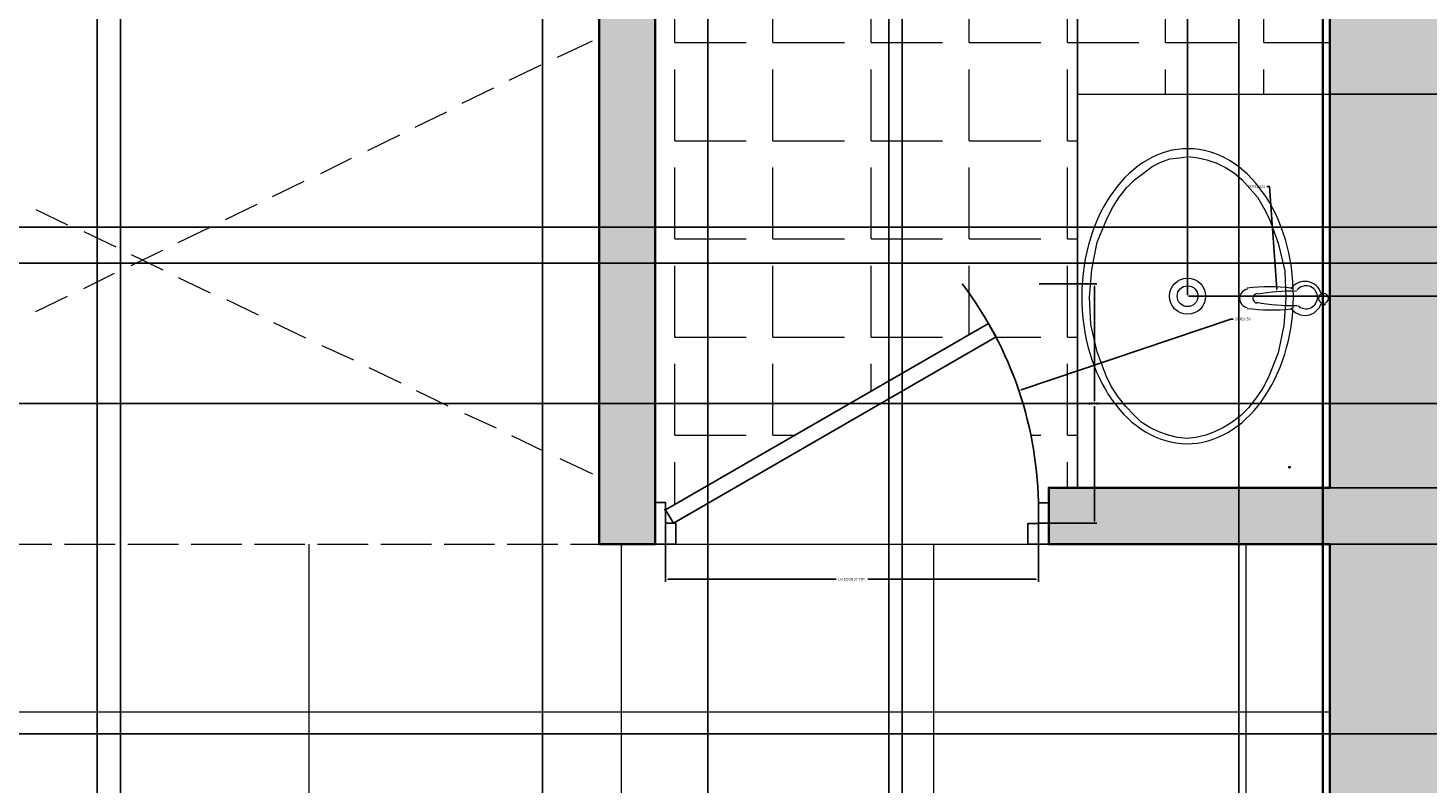
# Model space of a CAD drawing. Units: inches. Extents: x 6 to 575, y 34 to 566.
# Tile 17 of 21: x 282 to 382, y 432 to 486. Entities that reach past the tile are written whole.
import ezdxf

# ---------------------------------------------------------------- set-up
doc = ezdxf.new("R2010")
doc.units = ezdxf.units.IN
doc.linetypes.add('ACAD_ISO02W100', pattern=[15, 12, -3])
for name, color, linetype, lineweight in [('A-ANNO-DIMS', 2, 'Continuous', 18), ('A-FLOR-CASE', 2, 'Continuous', 18), ('A-FLOR-FIXT', 9, 'Continuous', 18), ('A-FLOR-PATT', 252, 'Continuous', 9), ('A-FLOR-STRS-OVHD', 1, 'ACAD_ISO02W100', 13), ('A-WALL-PATT', 251, 'Continuous', 9), ('DOORS', 3, 'Continuous', 25), ('STAIRS', 1, 'Continuous', 20), ('WALLS', 7, 'Continuous', 35)]:
    doc.layers.add(name, color=color, linetype=linetype, lineweight=lineweight)
doc.styles.get("Standard").update_dxf_attribs({"font": 'arial.ttf'})
doc.dimstyles.get("Standard").update_dxf_attribs({"dimtxt": 0.18, "dimasz": 0.18, "dimexe": 0.18, "dimexo": 0.0625, "dimgap": 0.09, "dimtad": 0, "dimtih": 1, "dimtoh": 1, "dimdec": 4, "dimzin": 0, "dimdsep": 46, "dimtxsty": 'Standard', "dimcen": 0.09, "dimadec": 0, "dimazin": 0, "dimtfac": 1, "dimtdec": 4, "dimtofl": 0, "dimtmove": 0, "dimatfit": 3, "dimfxl": 1, "dimtolj": 1, "dimtzin": 0, "dimarcsym": 0})

# ---------------------------------------------------------------- blocks, each defined once
blk = doc.blocks.new('Door - Left Hung 36 in.')
blk.add_lwpolyline([(0.75, -1.3), (0, 0), (31.18, 18), (31.93, 16.7)], close=True)
blk.add_arc((0, 0), 36, 0, 37.3101)
blk = doc.blocks.new('*D13')
at = {"layer": 'A-ANNO-DIMS', "color": 0, "lineweight": -2, "transparency": 16777216}
for p, q in [((327.396, 450.212), (327.396, 446.115)), ((353.927, 450.212), (353.927, 446.115)), ((327.576, 446.295), (339.529, 446.295)), ((353.747, 446.295), (341.793, 446.295))]:
    blk.add_line(p, q, dxfattribs=at)
at = {"layer": 'A-ANNO-DIMS', "color": 0, "transparency": 16777216}
for points in [[(327.576, 446.325), (327.576, 446.265), (327.396, 446.295)], [(353.747, 446.325), (353.747, 446.265), (353.927, 446.295)]]:
    blk.add_solid(points, dxfattribs=at)
at = {"layer": 'Defpoints', "color": 0, "transparency": 16777216}
for p in [(327.396, 450.275), (353.927, 450.275), (353.927, 446.295)]:
    blk.add_point(p, dxfattribs=at)
at = {"layer": 'A-ANNO-DIMS', "color": 0, "transparency": 16777216, "insert": (340.661, 446.295), "char_height": 0.18, "attachment_point": 5}
blk.add_mtext('\\A1;LH DOOR 27 TYP.', dxfattribs=at)
blk = doc.blocks.new('*D14')
at = {"layer": 'A-ANNO-DIMS', "color": 0, "lineweight": -2, "transparency": 16777216}
for p, q in [((353.989, 467.313), (358.086, 467.313)), ((357.906, 467.133), (357.906, 458.975)), ((357.906, 450.455), (357.906, 458.614)), ((353.989, 450.275), (358.086, 450.275))]:
    blk.add_line(p, q, dxfattribs=at)
at = {"layer": 'A-ANNO-DIMS', "color": 0, "transparency": 16777216}
for points in [[(357.876, 467.133), (357.936, 467.133), (357.906, 467.313)], [(357.876, 450.455), (357.936, 450.455), (357.906, 450.275)]]:
    blk.add_solid(points, dxfattribs=at)
at = {"layer": 'Defpoints', "color": 0, "transparency": 16777216}
for p in [(353.927, 467.313), (357.906, 467.313), (353.927, 450.275)]:
    blk.add_point(p, dxfattribs=at)
at = {"layer": 'A-ANNO-DIMS', "color": 0, "transparency": 16777216, "insert": (357.906, 458.794), "char_height": 0.18, "attachment_point": 5}
blk.add_mtext('\\A1;17 TYP.', dxfattribs=at)
blk = doc.blocks.new('*D50')
at = {"layer": 'A-ANNO-DIMS', "color": 0, "lineweight": -2, "transparency": 16777216}
for p, q in [((248.696, 468.775), (574.676, 468.775)), ((574.496, 468.595), (574.496, 463.964)), ((574.496, 458.969), (574.496, 463.6)), ((248.696, 458.789), (574.676, 458.789))]:
    blk.add_line(p, q, dxfattribs=at)
at = {"layer": 'A-ANNO-DIMS', "color": 0, "transparency": 16777216}
for points in [[(574.466, 468.595), (574.526, 468.595), (574.496, 468.775)], [(574.466, 458.969), (574.526, 458.969), (574.496, 458.789)]]:
    blk.add_solid(points, dxfattribs=at)
at = {"layer": 'Defpoints', "color": 0, "transparency": 16777216}
for p in [(248.633, 468.775), (574.496, 468.775), (248.633, 458.789)]:
    blk.add_point(p, dxfattribs=at)
at = {"layer": 'A-ANNO-DIMS', "color": 0, "transparency": 16777216, "insert": (574.496, 463.782), "char_height": 0.18, "attachment_point": 5}
blk.add_mtext('\\A1;9.987', dxfattribs=at)
blk = doc.blocks.new('*D52')
at = {"layer": 'A-ANNO-DIMS', "color": 0, "lineweight": -2, "transparency": 16777216}
for p, q in [((437.624, 471.353), (6.649, 471.353)), ((6.829, 471.173), (6.829, 453.513)), ((6.829, 435.488), (6.829, 453.149)), ((437.624, 435.308), (6.649, 435.308))]:
    blk.add_line(p, q, dxfattribs=at)
at = {"layer": 'A-ANNO-DIMS', "color": 0, "transparency": 16777216}
for points in [[(6.799, 471.173), (6.859, 471.173), (6.829, 471.353)], [(6.799, 435.488), (6.859, 435.488), (6.829, 435.308)]]:
    blk.add_solid(points, dxfattribs=at)
at = {"layer": 'Defpoints', "color": 0, "transparency": 16777216}
for p in [(6.829, 471.353), (437.687, 471.353), (437.687, 435.308)]:
    blk.add_point(p, dxfattribs=at)
at = {"layer": 'A-ANNO-DIMS', "color": 0, "transparency": 16777216, "insert": (6.829, 453.331), "char_height": 0.18, "attachment_point": 5}
blk.add_mtext('\\A1;36.045', dxfattribs=at)
blk = doc.blocks.new('*D63')
at = {"layer": 'A-ANNO-DIMS', "color": 0, "lineweight": -2, "transparency": 16777216}
for p, q in [((322.659, 448.863), (322.659, 565.811)), ((322.839, 565.631), (324.506, 565.631)), ((326.479, 565.631), (324.811, 565.631)), ((326.659, 448.863), (326.659, 565.811))]:
    blk.add_line(p, q, dxfattribs=at)
at = {"layer": 'A-ANNO-DIMS', "color": 0, "transparency": 16777216}
for points in [[(322.839, 565.661), (322.839, 565.601), (322.659, 565.631)], [(326.479, 565.661), (326.479, 565.601), (326.659, 565.631)]]:
    blk.add_solid(points, dxfattribs=at)
at = {"layer": 'Defpoints', "color": 0, "transparency": 16777216}
for p in [(326.659, 565.631), (322.659, 448.801), (326.659, 448.801)]:
    blk.add_point(p, dxfattribs=at)
at = {"layer": 'A-ANNO-DIMS', "color": 0, "transparency": 16777216, "insert": (324.659, 565.631), "char_height": 0.18, "attachment_point": 5}
blk.add_mtext('\\A1;4', dxfattribs=at)
blk = doc.blocks.new('*D64')
at = {"layer": 'A-ANNO-DIMS', "color": 0, "lineweight": -2, "transparency": 16777216}
for p, q in [((354.721145, 452.800984), (574.675816, 452.800984)), ((574.495816, 452.620984), (574.495816, 450.980984)), ((574.495816, 448.980984), (574.495816, 450.620984)), ((354.721145, 448.800984), (574.675816, 448.800984))]:
    blk.add_line(p, q, dxfattribs=at)
at = {"layer": 'A-ANNO-DIMS', "color": 0, "transparency": 16777216}
for points in [[(574.465816, 452.620984), (574.525816, 452.620984), (574.495816, 452.800984)], [(574.465816, 448.980984), (574.525816, 448.980984), (574.495816, 448.800984)]]:
    blk.add_solid(points, dxfattribs=at)
at = {"layer": 'Defpoints', "color": 0, "transparency": 16777216}
for p in [(354.658645, 452.800984), (574.495816, 452.800984), (354.658645, 448.800984)]:
    blk.add_point(p, dxfattribs=at)
at = {"layer": 'A-ANNO-DIMS', "color": 0, "transparency": 16777216, "insert": (574.495816, 450.800984), "char_height": 0.18, "attachment_point": 5}
blk.add_mtext('\\A1;4', dxfattribs=at)
blk = doc.blocks.new('*D73')
at = {"layer": 'A-ANNO-DIMS', "color": 0, "lineweight": -2, "transparency": 16777216}
for p, q in [((248.633, 448.865), (248.633, 565.811)), ((248.813, 565.631), (285.253, 565.631)), ((322.479, 565.631), (286.039, 565.631)), ((322.659, 448.863), (322.659, 565.811))]:
    blk.add_line(p, q, dxfattribs=at)
at = {"layer": 'A-ANNO-DIMS', "color": 0, "transparency": 16777216}
for points in [[(248.813, 565.661), (248.813, 565.601), (248.633, 565.631)], [(322.479, 565.661), (322.479, 565.601), (322.659, 565.631)]]:
    blk.add_solid(points, dxfattribs=at)
at = {"layer": 'Defpoints', "color": 0, "transparency": 16777216}
for p in [(322.659, 565.631), (248.633, 448.802), (322.659, 448.801)]:
    blk.add_point(p, dxfattribs=at)
at = {"layer": 'A-ANNO-DIMS', "color": 0, "transparency": 16777216, "insert": (285.646, 565.631), "char_height": 0.18, "attachment_point": 5}
blk.add_mtext('\\A1;74.03', dxfattribs=at)
blk = doc.blocks.new('*D119')
at = {"layer": 'A-ANNO-DIMS', "color": 0, "lineweight": -2, "transparency": 16777216}
for p, q in [((343.278, 400.02), (343.278, 565.811)), ((343.458, 565.631), (358.358, 565.631)), ((374.011, 565.631), (359.111, 565.631)), ((374.191, 395.441), (374.191, 565.811))]:
    blk.add_line(p, q, dxfattribs=at)
at = {"layer": 'A-ANNO-DIMS', "color": 0, "transparency": 16777216}
for points in [[(343.458, 565.661), (343.458, 565.601), (343.278, 565.631)], [(374.011, 565.661), (374.011, 565.601), (374.191, 565.631)]]:
    blk.add_solid(points, dxfattribs=at)
at = {"layer": 'Defpoints', "color": 0, "transparency": 16777216}
for p in [(374.191, 565.631), (343.278, 399.958), (374.191, 395.379)]:
    blk.add_point(p, dxfattribs=at)
at = {"layer": 'A-ANNO-DIMS', "color": 0, "transparency": 16777216, "insert": (358.734, 565.631), "char_height": 0.18, "attachment_point": 5}
blk.add_mtext('\\A1;30.91', dxfattribs=at)
blk = doc.blocks.new('*D126')
at = {"layer": 'A-ANNO-DIMS', "color": 0, "lineweight": -2, "transparency": 16777216}
for p, q in [((368.183, 318.514), (368.183, 565.811)), ((368.363, 565.631), (370.782, 565.631)), ((373.954, 565.631), (371.535, 565.631)), ((374.134, 318.458), (374.134, 565.811))]:
    blk.add_line(p, q, dxfattribs=at)
at = {"layer": 'A-ANNO-DIMS', "color": 0, "transparency": 16777216}
for points in [[(368.363, 565.661), (368.363, 565.601), (368.183, 565.631)], [(373.954, 565.661), (373.954, 565.601), (374.134, 565.631)]]:
    blk.add_solid(points, dxfattribs=at)
at = {"layer": 'Defpoints', "color": 0, "transparency": 16777216}
for p in [(374.134, 565.631), (368.183, 318.451), (374.134, 318.395)]:
    blk.add_point(p, dxfattribs=at)
at = {"layer": 'A-ANNO-DIMS', "color": 0, "transparency": 16777216, "insert": (371.158, 565.631), "char_height": 0.18, "attachment_point": 5}
blk.add_mtext('\\A1;5.951', dxfattribs=at)
blk = doc.blocks.new('*D127')
at = {"layer": 'A-ANNO-DIMS', "color": 0, "lineweight": -2, "transparency": 16777216}
for p, q in [((286.946, 310.606), (286.946, 565.811)), ((287.126, 565.631), (308.278, 565.631)), ((330.225, 565.631), (309.073, 565.631)), ((330.405, 310.606), (330.405, 565.811))]:
    blk.add_line(p, q, dxfattribs=at)
at = {"layer": 'A-ANNO-DIMS', "color": 0, "transparency": 16777216}
for points in [[(287.126, 565.661), (287.126, 565.601), (286.946, 565.631)], [(330.225, 565.661), (330.225, 565.601), (330.405, 565.631)]]:
    blk.add_solid(points, dxfattribs=at)
at = {"layer": 'Defpoints', "color": 0, "transparency": 16777216}
for p in [(330.405, 565.631), (286.946, 310.543), (330.405, 310.543)]:
    blk.add_point(p, dxfattribs=at)
at = {"layer": 'A-ANNO-DIMS', "color": 0, "transparency": 16777216, "insert": (308.675, 565.631), "char_height": 0.18, "attachment_point": 5}
blk.add_mtext('\\A1;43.46', dxfattribs=at)
blk = doc.blocks.new('*D129')
at = {"layer": 'A-ANNO-DIMS', "color": 0, "lineweight": -2, "transparency": 16777216}
for p, q in [((330.405, 310.606), (330.405, 565.811)), ((330.585, 565.631), (336.387, 565.631)), ((343.098, 565.631), (337.296, 565.631)), ((343.278, 313.883), (343.278, 565.811))]:
    blk.add_line(p, q, dxfattribs=at)
at = {"layer": 'A-ANNO-DIMS', "color": 0, "transparency": 16777216}
for points in [[(330.585, 565.661), (330.585, 565.601), (330.405, 565.631)], [(343.098, 565.661), (343.098, 565.601), (343.278, 565.631)]]:
    blk.add_solid(points, dxfattribs=at)
at = {"layer": 'Defpoints', "color": 0, "transparency": 16777216}
for p in [(343.278, 565.631), (343.278, 313.82), (330.405, 310.543)]:
    blk.add_point(p, dxfattribs=at)
at = {"layer": 'A-ANNO-DIMS', "color": 0, "transparency": 16777216, "insert": (336.841, 565.631), "char_height": 0.18, "attachment_point": 5}
blk.add_mtext('\\A1;12.874', dxfattribs=at)
blk = doc.blocks.new('*D131')
at = {"layer": 'A-ANNO-DIMS', "color": 0, "lineweight": -2, "transparency": 16777216}
for p, q in [((288.603, 342.076), (288.603, 565.811)), ((288.783, 565.631), (303.229, 565.631)), ((318.461, 565.631), (304.015, 565.631)), ((318.641, 342.076), (318.641, 565.811))]:
    blk.add_line(p, q, dxfattribs=at)
at = {"layer": 'A-ANNO-DIMS', "color": 0, "transparency": 16777216}
for points in [[(288.783, 565.661), (288.783, 565.601), (288.603, 565.631)], [(318.461, 565.661), (318.461, 565.601), (318.641, 565.631)]]:
    blk.add_solid(points, dxfattribs=at)
at = {"layer": 'Defpoints', "color": 0, "transparency": 16777216}
for p in [(318.641, 565.631), (288.603, 342.013), (318.641, 342.013)]:
    blk.add_point(p, dxfattribs=at)
at = {"layer": 'A-ANNO-DIMS', "color": 0, "transparency": 16777216, "insert": (303.622, 565.631), "char_height": 0.18, "attachment_point": 5}
blk.add_mtext('\\A1;30.04', dxfattribs=at)
blk = doc.blocks.new('*D134')
at = {"layer": 'A-ANNO-DIMS', "color": 0, "lineweight": -2, "transparency": 16777216}
for p, q in [((318.641, 342.076), (318.641, 565.811)), ((318.821, 565.631), (331.04, 565.631)), ((344.051, 565.631), (331.831, 565.631)), ((344.231, 343.012), (344.231, 565.811))]:
    blk.add_line(p, q, dxfattribs=at)
at = {"layer": 'A-ANNO-DIMS', "color": 0, "transparency": 16777216}
for points in [[(318.821, 565.661), (318.821, 565.601), (318.641, 565.631)], [(344.051, 565.661), (344.051, 565.601), (344.231, 565.631)]]:
    blk.add_solid(points, dxfattribs=at)
at = {"layer": 'Defpoints', "color": 0, "transparency": 16777216}
for p in [(344.231, 565.631), (344.231, 342.949), (318.641, 342.013)]:
    blk.add_point(p, dxfattribs=at)
at = {"layer": 'A-ANNO-DIMS', "color": 0, "transparency": 16777216, "insert": (331.436, 565.631), "char_height": 0.18, "attachment_point": 5}
blk.add_mtext('\\A1;25.59', dxfattribs=at)
blk = doc.blocks.new('*D193')
at = {"layer": 'A-ANNO-DIMS', "color": 0, "lineweight": -2, "transparency": 16777216}
for p, q in [((356.714, 452.863), (356.714, 565.811)), ((356.894, 565.631), (365.231, 565.631)), ((374.479, 565.631), (366.142, 565.631)), ((374.659, 480.873), (374.659, 565.811))]:
    blk.add_line(p, q, dxfattribs=at)
at = {"layer": 'A-ANNO-DIMS', "color": 0, "transparency": 16777216}
for points in [[(356.894, 565.661), (356.894, 565.601), (356.714, 565.631)], [(374.479, 565.661), (374.479, 565.601), (374.659, 565.631)]]:
    blk.add_solid(points, dxfattribs=at)
at = {"layer": 'Defpoints', "color": 0, "transparency": 16777216}
for p in [(374.659, 565.631), (374.659, 480.81), (356.714, 452.801)]:
    blk.add_point(p, dxfattribs=at)
at = {"layer": 'A-ANNO-DIMS', "color": 0, "transparency": 16777216, "insert": (365.686, 565.631), "char_height": 0.18, "attachment_point": 5}
blk.add_mtext('\\A1;17.945', dxfattribs=at)
blk = doc.blocks.new('*D194')
at = {"layer": 'A-ANNO-DIMS', "color": 0, "lineweight": -2, "transparency": 16777216}
for p, q in [((374.721, 480.81), (574.676, 480.81)), ((574.496, 480.63), (574.496, 466.987)), ((574.496, 452.981), (574.496, 466.624)), ((356.777, 452.801), (574.676, 452.801))]:
    blk.add_line(p, q, dxfattribs=at)
at = {"layer": 'A-ANNO-DIMS', "color": 0, "transparency": 16777216}
for points in [[(574.466, 480.63), (574.526, 480.63), (574.496, 480.81)], [(574.466, 452.981), (574.526, 452.981), (574.496, 452.801)]]:
    blk.add_solid(points, dxfattribs=at)
at = {"layer": 'Defpoints', "color": 0, "transparency": 16777216}
for p in [(374.659, 480.81), (574.496, 480.81), (356.714, 452.801)]:
    blk.add_point(p, dxfattribs=at)
at = {"layer": 'A-ANNO-DIMS', "color": 0, "transparency": 16777216, "insert": (574.496, 466.806), "char_height": 0.18, "attachment_point": 5}
blk.add_mtext('\\A1;28.01', dxfattribs=at)
blk = doc.blocks.new('*D195')
at = {"layer": 'A-ANNO-DIMS', "color": 0, "lineweight": -2, "transparency": 16777216}
for p, q in [((364.602, 466.433), (574.676, 466.433)), ((574.496, 466.253), (574.496, 459.799)), ((574.496, 452.981), (574.496, 459.435)), ((374.721, 452.801), (574.676, 452.801))]:
    blk.add_line(p, q, dxfattribs=at)
at = {"layer": 'A-ANNO-DIMS', "color": 0, "transparency": 16777216}
for points in [[(574.466, 466.253), (574.526, 466.253), (574.496, 466.433)], [(574.466, 452.981), (574.526, 452.981), (574.496, 452.801)]]:
    blk.add_solid(points, dxfattribs=at)
at = {"layer": 'Defpoints', "color": 0, "transparency": 16777216}
for p in [(364.54, 466.433), (574.496, 466.433), (374.659, 452.801)]:
    blk.add_point(p, dxfattribs=at)
at = {"layer": 'A-ANNO-DIMS', "color": 0, "transparency": 16777216, "insert": (574.496, 459.617), "char_height": 0.18, "attachment_point": 5}
blk.add_mtext('\\A1;13.632', dxfattribs=at)
blk = doc.blocks.new('*D196')
at = {"layer": 'A-ANNO-DIMS', "color": 0, "lineweight": -2, "transparency": 16777216}
for p, q in [((364.54, 466.496), (364.54, 565.811)), ((364.72, 565.631), (369.215, 565.631)), ((374.479, 565.631), (369.983, 565.631)), ((374.659, 452.863), (374.659, 565.811))]:
    blk.add_line(p, q, dxfattribs=at)
at = {"layer": 'A-ANNO-DIMS', "color": 0, "transparency": 16777216}
for points in [[(364.72, 565.661), (364.72, 565.601), (364.54, 565.631)], [(374.479, 565.661), (374.479, 565.601), (374.659, 565.631)]]:
    blk.add_solid(points, dxfattribs=at)
at = {"layer": 'Defpoints', "color": 0, "transparency": 16777216}
for p in [(364.54, 565.631), (364.54, 466.433), (374.659, 452.801)]:
    blk.add_point(p, dxfattribs=at)
at = {"layer": 'A-ANNO-DIMS', "color": 0, "transparency": 16777216, "insert": (369.599, 565.631), "char_height": 0.18, "attachment_point": 5}
blk.add_mtext('\\A1;10.12', dxfattribs=at)
blk = doc.blocks.new('*D230')
at = {"layer": 'A-ANNO-DIMS', "color": 0, "lineweight": -2, "transparency": 16777216}
for p, q in [((367.615, 464.811), (352.703, 459.776)), ((367.795, 464.811), (367.615, 464.811)), ((327.396, 451.142), (327.396, 451.322)), ((327.306, 451.232), (327.486, 451.232))]:
    blk.add_line(p, q, dxfattribs=at)
at = {"layer": 'A-ANNO-DIMS', "color": 0, "transparency": 16777216}
blk.add_solid([(352.694, 459.805), (352.713, 459.748), (352.533, 459.719)], dxfattribs=at)
at = {"layer": 'Defpoints', "color": 0, "transparency": 16777216}
for p in [(352.533, 459.719), (327.396, 451.232)]:
    blk.add_point(p, dxfattribs=at)
at = {"layer": 'A-ANNO-DIMS', "color": 0, "transparency": 16777216, "insert": (368.47, 464.811), "char_height": 0.18, "attachment_point": 5}
blk.add_mtext('\\A1;2X R26.53', dxfattribs=at)
blk = doc.blocks.new('*D233')
at = {"layer": 'A-ANNO-DIMS', "color": 0, "lineweight": -2, "transparency": 16777216}
for p, q in [((370.184, 474.246), (370.364, 474.246)), ((370.364, 474.246), (370.888, 466.931)), ((371.796, 454.172), (371.796, 454.352)), ((371.706, 454.262), (371.886, 454.262))]:
    blk.add_line(p, q, dxfattribs=at)
at = {"layer": 'A-ANNO-DIMS', "color": 0, "transparency": 16777216}
blk.add_solid([(370.918, 466.934), (370.858, 466.929), (370.901, 466.752)], dxfattribs=at)
at = {"layer": 'Defpoints', "color": 0, "transparency": 16777216}
for p in [(370.901, 466.752), (371.796, 454.262)]:
    blk.add_point(p, dxfattribs=at)
at = {"layer": 'A-ANNO-DIMS', "color": 0, "transparency": 16777216, "insert": (369.44, 474.246), "char_height": 0.18, "attachment_point": 5}
blk.add_mtext('\\A1;2X R12.522', dxfattribs=at)

msp = doc.modelspace()

# ---------------------------------------------------------------- hatches: boundary and pattern name
at = {"layer": 'A-FLOR-PATT'}
h = msp.add_hatch(dxfattribs=at)
h.set_pattern_fill('ANGLE', color=256)
h.set_pattern_definition([(0, (-98.035, 170.1465), (0, 6.985), [5.08, -1.905]), (90, (-98.035, 170.1465), (-6.985, 4e-16), [5.08, -1.905])])
h.paths.add_polyline_path([(374.6586, 530.801), (362.6586, 530.801), (338.6586, 530.801), (326.6586, 530.801), (326.6586, 451.7489), (327.3956, 451.7489), (327.3956, 451.2323), (350.3721, 464.4978), (350.9248, 463.5404), (350.9049, 463.5289, -0.1161983), (353.9217, 451.7417), (354.6586, 451.7417), (354.6586, 452.801), (356.7141, 452.801), (356.7141, 480.81), (374.6586, 480.81)])
h = msp.add_hatch(dxfattribs=at)
h.set_pattern_fill('NET', color=256, scale=7)
h.set_pattern_definition([(0, (-98.035, 170.147), (0, 22.225), []), (90, (-98.035, 170.147), (-22.225, 1e-15), [])])
h.paths.add_polyline_path([(368.183, 395.6385, -0.8837053), (374.2533, 394.8861), (374.6586, 448.801), (354.6586, 448.801), (354.6586, 448.7938), (353.1847, 448.7938), (326.6586, 448.801), (322.6586, 448.801), (248.6332, 448.8024), (206.6586, 448.8024), (206.6586, 389.449), (221.6622, 389.449), (221.6622, 310.5712), (206.6586, 310.5712), (206.6586, 276.801), (206.6704, 276.801), (206.6704, 274.3795), (206.6586, 224.801), (246.6586, 224.801), (264.6586, 224.801), (265.6986, 224.801), (265.6986, 249.081), (267.5186, 249.081), (267.5186, 249.0145, -0.3851529), (290.6494, 224.801), (290.6679, 224.801, -0.3851529), (313.7986, 249.0145), (313.7986, 249.081), (315.6186, 249.081), (315.6186, 224.801), (316.6586, 224.801), (334.6586, 224.801), (374.6586, 224.801), (374.6586, 278.801), (374.1753, 318.8919, -0.4553029), (370.7577, 315.9168), (370.6643, 313.8205, -0.4142136), (368.7528, 311.909), (368.8072, 311.8975), (368.7528, 311.909, 0.4142136), (370.6643, 313.8205), (370.7632, 315.9161, -0.346346), (368.183, 318.5897)])
h.paths.add_polyline_path([(288.603, 342.0131), (288.603, 389.9952), (318.6406, 389.9952), (318.6406, 342.0131)], flags=16)
h.paths.add_polyline_path([(289.6173, 343.0274), (289.6173, 389.059), (317.6263, 389.059), (317.6263, 343.0274)], flags=0)
h.paths.add_polyline_path([(295.4867, 311.7535, 0.0653816), (295.1241, 312.0945), (295.0006, 312.1316)], flags=16)
h.paths.add_polyline_path([(328.4931, 284.9911, 0.4142136), (330.4045, 286.9026), (330.4215, 286.8532), (330.4045, 286.9026, -0.4142136), (328.4931, 284.9911), (328.549, 284.9808)], flags=16)
h.paths.add_polyline_path([(344.7771, 305.2659), (368.8072, 305.2659), (368.8072, 281.2358), (344.7771, 281.2358)], flags=16)
h.paths.add_polyline_path([(368.183, 288.1406, -1), (356.246, 288.1406, -1)], flags=0)
h.paths.add_polyline_path([(347.9759, 404.6629), (347.9759, 428.6929), (372.006, 428.6929), (372.006, 404.6629)], flags=16)
h.paths.add_polyline_path([(359.4448, 421.7882, -1), (371.3818, 421.7882, -1)], flags=0)
at = {"layer": 'A-WALL-PATT'}
h = msp.add_hatch(color=256, dxfattribs=at)
h.dxf.hatch_style = 1
h.paths.add_polyline_path([(160.6586, 539.801), (32.6586, 539.801), (32.6586, 272.801), (41.6586, 272.801), (41.6586, 286.0643), (41.6586, 358.0764), (41.6586, 379.0637), (41.6586, 407.7709), (41.6194, 407.7709), (41.6194, 431.801), (82.8918, 431.801), (82.8918, 440.801), (65.6494, 440.801), (65.6494, 440.7732), (41.6194, 440.7732), (41.6194, 515.5941), (41.6586, 530.801), (117.6586, 530.801), (117.6586, 474.801), (120.6068, 474.801), (121.6586, 474.801), (121.6586, 530.801), (137.4275, 530.801), (137.4275, 530.8356), (141.2505, 530.8356), (160.6586, 530.801)])
h.paths.add_polyline_path([(71.6586, 212.801), (41.6586, 212.801), (41.6586, 224.801), (32.6586, 224.801), (32.6586, 203.801), (71.6586, 203.801)])
h.paths.add_polyline_path([(206.6586, 215.801), (246.6586, 215.801), (246.6586, 224.801), (206.6586, 224.801), (206.6586, 230.801), (201.8157, 230.801), (197.6586, 230.801), (197.6586, 212.801), (167.6586, 212.801), (167.6586, 203.801), (206.6586, 203.801)])
h.paths.add_polyline_path([(383.6586, 224.801), (334.6586, 224.801), (334.6586, 215.801), (374.6586, 215.801), (374.6586, 203.801), (384.0753, 203.801), (407.6586, 203.801), (407.6586, 212.801), (383.6586, 212.801)])
h.paths.add_polyline_path([(548.6586, 270.801), (539.6586, 270.801), (539.6586, 212.801), (515.6586, 212.801), (515.6586, 203.801), (548.6586, 203.801)])
h.paths.add_polyline_path([(548.6586, 412.801), (545.7108, 412.801), (539.6586, 412.801), (539.6586, 382.801), (433.708, 382.801), (433.708, 378.801), (539.6586, 378.801), (539.6586, 366.801), (548.6586, 366.801)])
h.paths.add_polyline_path([(548.6586, 539.801), (455.9436, 539.801), (455.9436, 530.801), (539.6586, 530.801), (539.6586, 440.801), (548.6586, 440.801)])
h.paths.add_polyline_path([(407.9436, 539.801), (362.6586, 539.801), (362.6586, 530.801), (374.6586, 530.801), (374.6586, 452.801), (354.6586, 452.801), (354.6586, 448.801), (374.6586, 448.801), (374.6586, 278.801), (383.6586, 278.801), (383.6586, 530.801), (407.9436, 530.801)])
h.paths.add_polyline_path([(338.6586, 539.801), (320.6586, 539.801), (320.6586, 530.801), (322.6586, 530.801), (322.6586, 448.801), (326.6586, 448.801), (326.6586, 530.801), (338.6586, 530.801)])
h.paths.add_polyline_path([(272.6586, 539.801), (184.6586, 539.801), (184.6586, 530.801), (197.6586, 530.801), (197.6586, 440.801), (176.6714, 440.801), (121.6586, 440.801), (121.6586, 446.801), (117.6586, 446.801), (117.6586, 440.801), (111.6586, 440.801), (111.6586, 431.801), (197.6586, 431.801), (197.6586, 407.7709), (197.6586, 276.801), (206.6586, 276.801), (206.6586, 530.801), (272.6586, 530.801)])

# ---------------------------------------------------------------- linework, layer by layer
at = {"layer": 'A-FLOR-CASE'}
msp.add_lwpolyline([(374.6586, 452.801), (356.7141, 452.801), (356.7141, 480.81), (374.6586, 480.81)], close=True, dxfattribs=at)
at = {"layer": 'A-FLOR-FIXT'}
msp.add_lwpolyline([(364.5941, 476.3629), (365.2963, 476.2849), (365.9204, 476.1289), (366.6226, 475.8948), (367.2468, 475.5827), (367.8709, 475.1926), (368.4171, 474.7245), (368.9632, 474.1003), (369.5093, 473.4762), (369.9775, 472.696), (370.3676, 471.9158), (370.9917, 470.1994), (371.4598, 468.2489), (371.5379, 466.2984), (371.3818, 464.3479), (370.9917, 462.3974), (370.2895, 460.681), (369.8994, 459.9008), (369.4313, 459.1986), (368.8852, 458.4964), (368.3391, 457.9503), (367.7149, 457.4822), (367.0907, 457.0921), (366.4666, 456.78), (365.8424, 456.5459), (365.1403, 456.3899), (364.5161, 456.3119), (363.8139, 456.3899), (363.1898, 456.5459), (362.4876, 456.78), (361.8634, 457.0921), (361.2393, 457.4822), (360.6931, 458.0283), (360.147, 458.5744), (359.6009, 459.2766), (359.1327, 459.9788), (358.7426, 460.759), (358.1185, 462.4754), (357.6504, 464.4259), (357.5723, 466.3764), (357.7284, 468.3269), (358.1185, 470.2774), (358.8207, 471.9938), (359.2108, 472.774), (359.6789, 473.4762), (360.225, 474.1784), (360.7712, 474.7245), (361.3953, 475.1926), (362.0195, 475.6607), (362.6436, 475.9728), (363.2678, 476.2069), (363.97, 476.2849)], close=True, dxfattribs=at)
for points in [[(374.3466, 466.6105), (374.1905, 466.6105)], [(374.3466, 465.8303), (374.1905, 465.8303)]]:
    msp.add_lwpolyline(points, dxfattribs=at)
for radius in [1.2873, 0.7412]:
    msp.add_circle((364.5396, 466.433), radius, dxfattribs=at)
for centre, radius, start, end in [((372.888, 466.277), 1.2093, 16.627786, 145.107366), ((368.9089, 466.277), 0.6632, 99.915126, 259.414585), ((370.3913, 453.0131), 14.0828, 83.798166, 96.553252), ((369.533, 466.277), 0.3511, 96.82233, 262.507381), ((371.7957, 454.2615), 12.5223, 87.687276, 100.502888), ((372.9661, 466.355), 0.8192, 224.664897, 142.421203), ((374.2144, 466.277), 0.3511, 99.909595, 259.420117), ((374.2144, 466.277), 0.3511, 279.909595, 79.420117), ((370.5473, 479.5409), 14.0828, 262.776459, 275.531545), ((371.8737, 478.2925), 12.5223, 258.826817, 271.977499), ((372.888, 466.277), 1.2093, 214.222345, 342.701926)]:
    msp.add_arc(centre, radius, start, end, dxfattribs=at)
for points in [[(364.601, 476.9267), (360.4429, 476.951), (357.0446, 472.2725), (357.0107, 466.4771)], [(372.0685, 466.389), (372.1024, 472.1845), (368.7591, 476.9023), (364.601, 476.9267)], [(357.0107, 466.4771), (356.9768, 460.6816), (360.3201, 455.9637), (364.4782, 455.9394)], [(364.4782, 455.9394), (368.6363, 455.9151), (372.0346, 460.5935), (372.0685, 466.389)]]:
    msp.add_open_spline(points, degree=3, dxfattribs=at)
at = {"layer": 'A-FLOR-STRS-OVHD', "ltscale": 0.3}
msp.add_line((248.6332, 448.8024), (322.6586, 448.8024), dxfattribs=at)
at = {"layer": 'A-FLOR-STRS-OVHD'}
for points in [[(319.7091, 483.4431), (322.2057, 484.6134)], [(316.2762, 481.8047), (318.5388, 482.8969)], [(312.9214, 480.1662), (315.1839, 481.2585)], [(309.5665, 478.4498), (311.8291, 479.5421)], [(306.2117, 476.8114), (308.4743, 477.9037)], [(302.8568, 475.173), (305.0414, 476.2653)], [(299.424, 473.5346), (301.6865, 474.6269)], [(282.5717, 472.5983), (284.8343, 471.5061)], [(296.0691, 471.8962), (298.3317, 472.9884)], [(292.7143, 470.2578), (294.9769, 471.35)], [(286.0046, 471.038), (288.2672, 469.9457)], [(289.3594, 468.6193), (291.622, 469.7116)], [(289.3594, 469.3995), (291.622, 468.3073)], [(286.0046, 466.9809), (288.1892, 468.0732)], [(292.7143, 467.7611), (294.9769, 466.6689)], [(282.5717, 465.3425), (284.8343, 466.4348)], [(296.1472, 466.2007), (298.4097, 465.1085)], [(299.502, 464.5623), (301.7646, 463.47)], [(302.9349, 462.9239), (305.1974, 461.9097)], [(306.2897, 461.3635), (308.5523, 460.2712)], [(309.6446, 459.7251), (311.9071, 458.6328)], [(313.0774, 458.0867), (315.34, 457.0724)], [(316.4323, 456.5263), (318.6948, 455.434)], [(319.8651, 454.8879), (322.2057, 453.7956)]]:
    msp.add_lwpolyline(points, dxfattribs=at)
at = {"layer": 'DOORS'}
for points in [[(326.6586, 448.801), (326.6586, 451.7489), (327.3956, 451.7489), (327.3956, 450.2749), (328.1326, 450.2749), (328.1326, 448.801)], [(354.6586, 448.7938), (354.6586, 451.7417), (353.9217, 451.7417), (353.9217, 450.2678), (353.1847, 450.2678), (353.1847, 448.7938)]]:
    msp.add_lwpolyline(points, close=True, dxfattribs=at)
at = {"layer": 'STAIRS'}
msp.add_line((322.6586, 448.801), (374.6586, 448.801), dxfattribs=at)
at = {"layer": 'WALLS'}
msp.add_line((374.6586, 278.801), (374.6586, 448.801), dxfattribs=at)
for points in [[(338.6586, 530.801), (326.6586, 530.801), (326.6586, 448.801), (322.6586, 448.801), (322.6586, 530.801)], [(374.6586, 448.801), (354.6586, 448.801), (354.6586, 452.801), (374.6586, 452.801), (374.6586, 530.801), (362.6586, 530.801)]]:
    msp.add_lwpolyline(points, dxfattribs=at)

# ---------------------------------------------------------------- block references
at = {"layer": 'DOORS', "xscale": 0.7369707940286806, "yscale": 0.7369707940286806, "zscale": 0.7369707940286806}
msp.add_blockref('Door - Left Hung 36 in.', (327.3956, 451.2323), dxfattribs=at)

# ---------------------------------------------------------------- dimensions: what is measured, and where the dimension line sits
at = {"layer": 'A-ANNO-DIMS'}
for base, p1, p2, override, picture, middle in [((322.6586, 565.631), (248.6332, 448.8024), (322.6586, 448.801), {"dimdec": 2, "dimlfac": 1, "dimrnd": 0, "dimzin": 0, "dimdsep": 46, "dimlunit": 2}, '*D73', (285.6459, 565.631)), ((330.4045, 565.631), (286.946, 310.5435), (330.4045, 310.5435), {"dimdec": 2, "dimlfac": 1, "dimrnd": 0, "dimzin": 0, "dimdsep": 46, "dimlunit": 2}, '*D127', (308.6753, 565.631)), ((318.6406, 565.631), (288.603, 342.0131), (318.6406, 342.0131), {"dimdec": 2, "dimlfac": 1, "dimrnd": 0, "dimzin": 0, "dimdsep": 46, "dimlunit": 2}, '*D131', (303.6218, 565.631)), ((344.231, 565.631), (318.6406, 342.0131), (344.231, 342.9494), {"dimdec": 2, "dimlfac": 1, "dimrnd": 0, "dimzin": 0, "dimdsep": 46, "dimlunit": 2}, '*D134', (331.4358, 565.631)), ((326.6586, 565.631), (322.6586, 448.801), (326.6586, 448.801), {"dimdec": 0, "dimlfac": 1, "dimrnd": 0, "dimzin": 0, "dimdsep": 46, "dimlunit": 2}, '*D63', (324.6586, 565.631)), ((343.2784, 565.631), (330.4045, 310.5435), (343.2784, 313.8205), {"dimdec": 3, "dimlfac": 1, "dimrnd": 0, "dimzin": 0, "dimdsep": 46, "dimlunit": 2}, '*D129', (336.8415, 565.631)), ((374.1905, 565.631), (343.2784, 399.9576), (374.1905, 395.3785), {"dimdec": 2, "dimlfac": 1, "dimrnd": 0, "dimzin": 0, "dimdsep": 46, "dimlunit": 2}, '*D119', (358.7345, 565.631)), ((374.65864, 565.63098), (356.71413, 452.80098), (374.65864, 480.81003), {"dimdec": 3, "dimlfac": 1, "dimrnd": 0, "dimzin": 0, "dimdsep": 46, "dimlunit": 2}, '*D193', (365.68639, 565.63098)), ((364.5396, 565.631), (374.6586, 452.801), (364.5396, 466.433), {"dimdec": 2, "dimlfac": 1, "dimrnd": 0, "dimzin": 0, "dimdsep": 46, "dimlunit": 2}, '*D196', (369.5991, 565.631)), ((374.134, 565.631), (368.183, 318.4512), (374.134, 318.3954), {"dimdec": 3, "dimlfac": 1, "dimrnd": 0, "dimzin": 0, "dimdsep": 46, "dimlunit": 2}, '*D126', (371.1585, 565.631))]:
    dim = msp.add_linear_dim(base=base, p1=p1, p2=p2, dimstyle='Standard', override=override, dxfattribs=at)
    dim.commit()
    dim.dimension.update_dxf_attribs({"geometry": picture, "text_midpoint": middle})
for base, p1, p2, override, picture, middle in [((574.4958, 480.81), (356.7141, 452.801), (374.6586, 480.81), {"dimdec": 2, "dimlfac": 1, "dimrnd": 0, "dimzin": 0, "dimdsep": 46, "dimlunit": 2}, '*D194', (574.4958, 466.8055)), ((6.8286, 471.3533), (437.687, 435.3082), (437.687, 471.3533), {"dimdec": 3, "dimlfac": 1, "dimrnd": 0, "dimzin": 0, "dimdsep": 46, "dimlunit": 2}, '*D52', (6.8286, 453.3307)), ((574.49582, 468.77538), (248.6332, 458.78887), (248.6332, 468.77538), {"dimdec": 3, "dimlfac": 1, "dimrnd": 0, "dimzin": 0, "dimdsep": 46, "dimlunit": 2}, '*D50', (574.49582, 463.78213)), ((574.4958, 466.433), (374.6586, 452.801), (364.5396, 466.433), {"dimdec": 3, "dimlfac": 1, "dimrnd": 0, "dimzin": 0, "dimdsep": 46, "dimlunit": 2}, '*D195', (574.4958, 459.617)), ((574.4958, 452.801), (354.6586, 448.801), (354.6586, 452.801), {"dimdec": 0, "dimlfac": 1, "dimrnd": 0, "dimzin": 0, "dimdsep": 46, "dimlunit": 2}, '*D64', (574.4958, 450.801))]:
    dim = msp.add_linear_dim(base=base, p1=p1, p2=p2, angle=90, dimstyle='Standard', override=override, dxfattribs=at)
    dim.commit()
    dim.dimension.update_dxf_attribs({"geometry": picture, "text_midpoint": middle})
for center, mpoint, override, picture, middle in [((371.7957, 454.2615), (370.901, 466.7518), {"dimdec": 3, "dimlfac": 1, "dimrnd": 0, "dimzin": 0, "dimdsep": 46, "dimlunit": 2}, '*D233', (369.4404, 474.246)), ((327.3956, 451.2323), (352.5326, 459.7189), {"dimdec": 2, "dimlfac": 1, "dimrnd": 0, "dimzin": 0, "dimdsep": 46, "dimlunit": 2}, '*D230', (368.4696, 464.8108))]:
    dim = msp.add_radius_dim(center=center, mpoint=mpoint, text='2X <>', dimstyle='Standard', override=override, dxfattribs=at)
    dim.commit()
    dim.dimension.update_dxf_attribs({"geometry": picture, "text_midpoint": middle, "dimtype": 164})
dim = msp.add_linear_dim(base=(357.9062, 467.3135), p1=(353.9266, 450.2749), p2=(353.9266, 467.3135), angle=90, text='<> TYP.', dimstyle='Standard', override={"dimdec": 0, "dimlfac": 1, "dimrnd": 0, "dimzin": 0, "dimdsep": 46, "dimlunit": 2}, dxfattribs=at)
dim.commit()
dim.dimension.update_dxf_attribs({"geometry": '*D14', "text_midpoint": (357.9062, 458.7942)})
dim = msp.add_linear_dim(base=(353.9266, 446.2953), p1=(327.3956, 450.2749), p2=(353.9266, 450.2749), text='LH DOOR <> TYP.', dimstyle='Standard', override={"dimdec": 0, "dimlfac": 1, "dimrnd": 0, "dimzin": 0, "dimdsep": 46, "dimlunit": 2}, dxfattribs=at)
dim.commit()
dim.dimension.update_dxf_attribs({"geometry": '*D13', "text_midpoint": (340.6611, 446.2953)})

doc.saveas('drawing.dxf')
